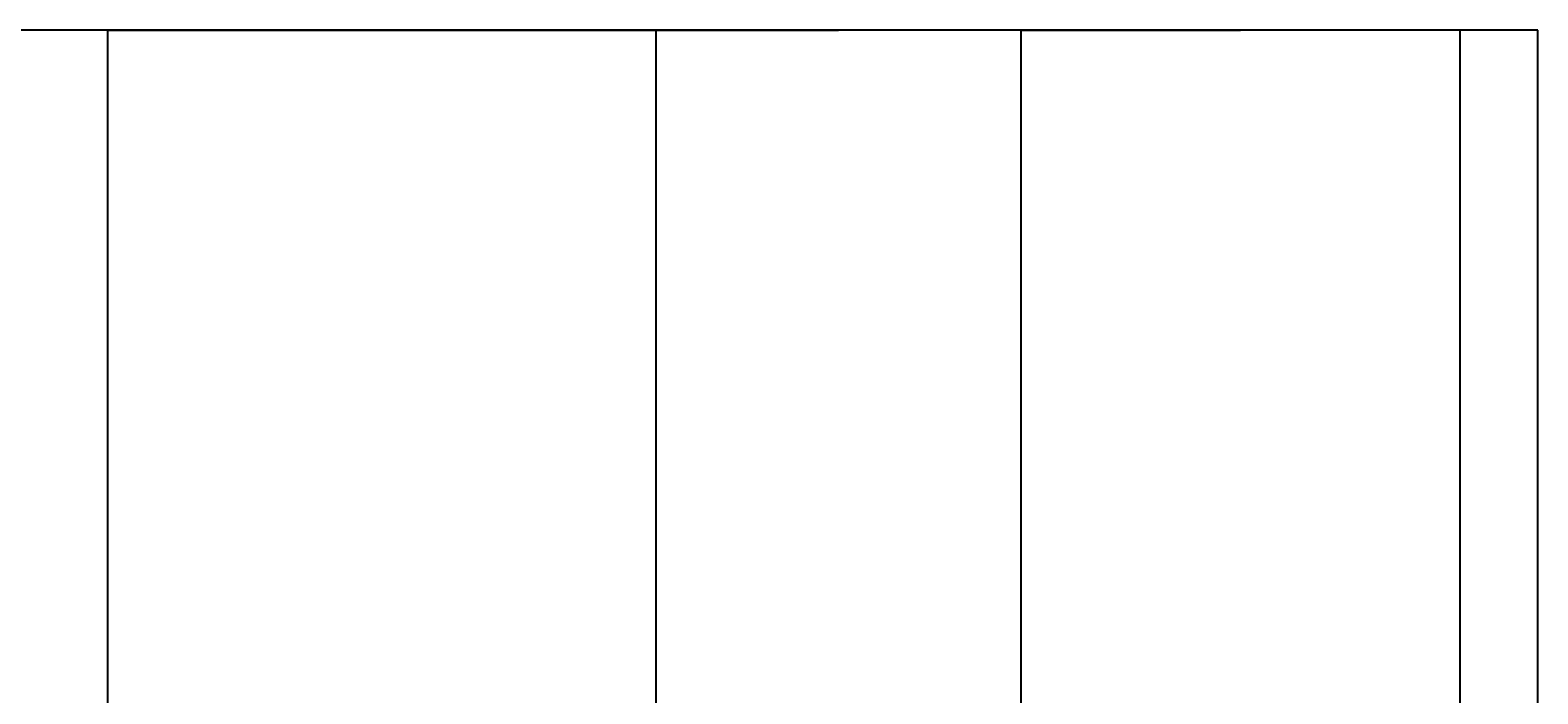
# Model space of a CAD drawing. Units: millimetres. Extents: x -229 to 16545, y -10488 to 4272.
# Tile 28 of 29: x 9556 to 14016, y 2307 to 4272. Entities that reach past the tile are written whole.
import ezdxf

# ---------------------------------------------------------------- set-up
doc = ezdxf.new("R2010")
doc.units = ezdxf.units.MM
doc.layers.add('A-ANNO-DIMS', color=2, linetype='Continuous', lineweight=18)
doc.styles.get("Standard").update_dxf_attribs({"font": 'arial.ttf'})
doc.dimstyles.get("Standard").update_dxf_attribs({"dimtxt": 0.18, "dimasz": 0.18, "dimexe": 0.18, "dimexo": 0.0625, "dimgap": 0.09, "dimtad": 0, "dimtih": 1, "dimtoh": 1, "dimdec": 4, "dimzin": 0, "dimdsep": 46, "dimtxsty": 'Standard', "dimcen": 0.09, "dimadec": 0, "dimazin": 0, "dimtfac": 1, "dimtdec": 4, "dimtofl": 0, "dimtmove": 0, "dimatfit": 3, "dimfxl": 1, "dimtolj": 1, "dimtzin": 0, "dimarcsym": 0})

# ---------------------------------------------------------------- blocks, each defined once
blk = doc.blocks.new('*D45')
at = {"layer": 'A-ANNO-DIMS', "color": 0, "lineweight": -2, "transparency": 16777216}
for p, q in [((2015.9, 2251.8), (2015.9, 4271.7)), ((2016.1, 4271.5), (8015.5, 4271.5)), ((14015.8, 4271.5), (8016.4, 4271.5)), ((14015.9, 2251.8), (14015.9, 4271.7))]:
    blk.add_line(p, q, dxfattribs=at)
at = {"layer": 'A-ANNO-DIMS', "color": 0, "transparency": 16777216}
for points in [[(2016.1, 4271.5), (2016.1, 4271.4), (2015.9, 4271.5)], [(14015.8, 4271.5), (14015.8, 4271.4), (14015.9, 4271.5)]]:
    blk.add_solid(points, dxfattribs=at)
at = {"layer": 'Defpoints', "color": 0, "transparency": 16777216}
for p in [(14015.9, 4271.5), (2015.9, 2251.7), (14015.9, 2251.7)]:
    blk.add_point(p, dxfattribs=at)
at = {"layer": 'A-ANNO-DIMS', "color": 0, "transparency": 16777216, "insert": (8015.9, 4271.5), "char_height": 0.18, "attachment_point": 5}
blk.add_mtext('\\A1;12000', dxfattribs=at)
blk = doc.blocks.new('*D52')
at = {"layer": 'A-ANNO-DIMS', "color": 0, "lineweight": -2, "transparency": 16777216}
for p, q in [((9785.9, -978.2), (9785.9, 4271.7)), ((9786.1, 4271.5), (11785.6, 4271.5)), ((13785.8, 4271.5), (11786.3, 4271.5)), ((13785.9, -978.2), (13785.9, 4271.7))]:
    blk.add_line(p, q, dxfattribs=at)
at = {"layer": 'A-ANNO-DIMS', "color": 0, "transparency": 16777216}
for points in [[(9786.1, 4271.5), (9786.1, 4271.4), (9785.9, 4271.5)], [(13785.8, 4271.5), (13785.8, 4271.4), (13785.9, 4271.5)]]:
    blk.add_solid(points, dxfattribs=at)
at = {"layer": 'Defpoints', "color": 0, "transparency": 16777216}
for p in [(13785.9, 4271.5), (9785.9, -978.3), (13785.9, -978.3)]:
    blk.add_point(p, dxfattribs=at)
at = {"layer": 'A-ANNO-DIMS', "color": 0, "transparency": 16777216, "insert": (11785.9, 4271.5), "char_height": 0.18, "attachment_point": 5}
blk.add_mtext('\\A1;4000', dxfattribs=at)
blk = doc.blocks.new('*D67')
at = {"layer": 'A-ANNO-DIMS', "color": 0, "lineweight": -2, "transparency": 16777216}
for p, q in [((11407.5, 2021.8), (11407.5, 4271.7)), ((11407.7, 4271.5), (11947.3, 4271.5)), ((12487.8, 4271.5), (11948.2, 4271.5)), ((12488, 2021.8), (12488, 4271.7))]:
    blk.add_line(p, q, dxfattribs=at)
at = {"layer": 'A-ANNO-DIMS', "color": 0, "transparency": 16777216}
for points in [[(11407.7, 4271.5), (11407.7, 4271.4), (11407.5, 4271.5)], [(12487.8, 4271.5), (12487.8, 4271.4), (12488, 4271.5)]]:
    blk.add_solid(points, dxfattribs=at)
at = {"layer": 'Defpoints', "color": 0, "transparency": 16777216}
for p in [(12488, 4271.5), (11407.5, 2021.7), (12488, 2021.7)]:
    blk.add_point(p, dxfattribs=at)
at = {"layer": 'A-ANNO-DIMS', "color": 0, "transparency": 16777216, "insert": (11947.8, 4271.5), "char_height": 0.18, "attachment_point": 5}
blk.add_mtext('\\A1;1080.5', dxfattribs=at)
blk = doc.blocks.new('*D68')
at = {"layer": 'A-ANNO-DIMS', "color": 0, "lineweight": -2, "transparency": 16777216}
for p, q in [((12488, 2021.8), (12488, 4271.7)), ((12488.2, 4271.5), (13136.6, 4271.5)), ((13785.8, 4271.5), (13137.3, 4271.5)), ((13785.9, 2021.8), (13785.9, 4271.7))]:
    blk.add_line(p, q, dxfattribs=at)
at = {"layer": 'A-ANNO-DIMS', "color": 0, "transparency": 16777216}
for points in [[(12488.2, 4271.5), (12488.2, 4271.4), (12488, 4271.5)], [(13785.8, 4271.5), (13785.8, 4271.4), (13785.9, 4271.5)]]:
    blk.add_solid(points, dxfattribs=at)
at = {"layer": 'Defpoints', "color": 0, "transparency": 16777216}
for p in [(13785.9, 4271.5), (12488, 2021.7), (13785.9, 2021.7)]:
    blk.add_point(p, dxfattribs=at)
at = {"layer": 'A-ANNO-DIMS', "color": 0, "transparency": 16777216, "insert": (13137, 4271.5), "char_height": 0.18, "attachment_point": 5}
blk.add_mtext('\\A1;1298', dxfattribs=at)

msp = doc.modelspace()

# ---------------------------------------------------------------- dimensions: what is measured, and where the dimension line sits
at = {"layer": 'A-ANNO-DIMS'}
for base, p1, p2, override, picture, middle in [((14015.933, 4271.479), (2015.933, 2251.728), (14015.933, 2251.728), {"dimdec": 0, "dimlfac": 1, "dimrnd": 0, "dimzin": 0, "dimdsep": 46, "dimlunit": 2}, '*D45', (8015.933, 4271.479)), ((13785.933, 4271.479), (9785.933, -978.272), (13785.933, -978.272), {"dimdec": 0, "dimlfac": 1, "dimrnd": 0, "dimzin": 0, "dimdsep": 46, "dimlunit": 2}, '*D52', (11785.933, 4271.479)), ((12488.002, 4271.479), (11407.51, 2021.728), (12488.002, 2021.728), {"dimdec": 1, "dimlfac": 1, "dimrnd": 0, "dimzin": 0, "dimdsep": 46, "dimlunit": 2}, '*D67', (11947.756, 4271.479)), ((13785.933, 4271.479), (12488.002, 2021.728), (13785.933, 2021.728), {"dimdec": 0, "dimlfac": 1, "dimrnd": 0, "dimzin": 0, "dimdsep": 46, "dimlunit": 2}, '*D68', (13136.967, 4271.479))]:
    dim = msp.add_linear_dim(base=base, p1=p1, p2=p2, dimstyle='Standard', override=override, dxfattribs=at)
    dim.commit()
    dim.dimension.update_dxf_attribs({"geometry": picture, "text_midpoint": middle})

doc.saveas('drawing.dxf')
